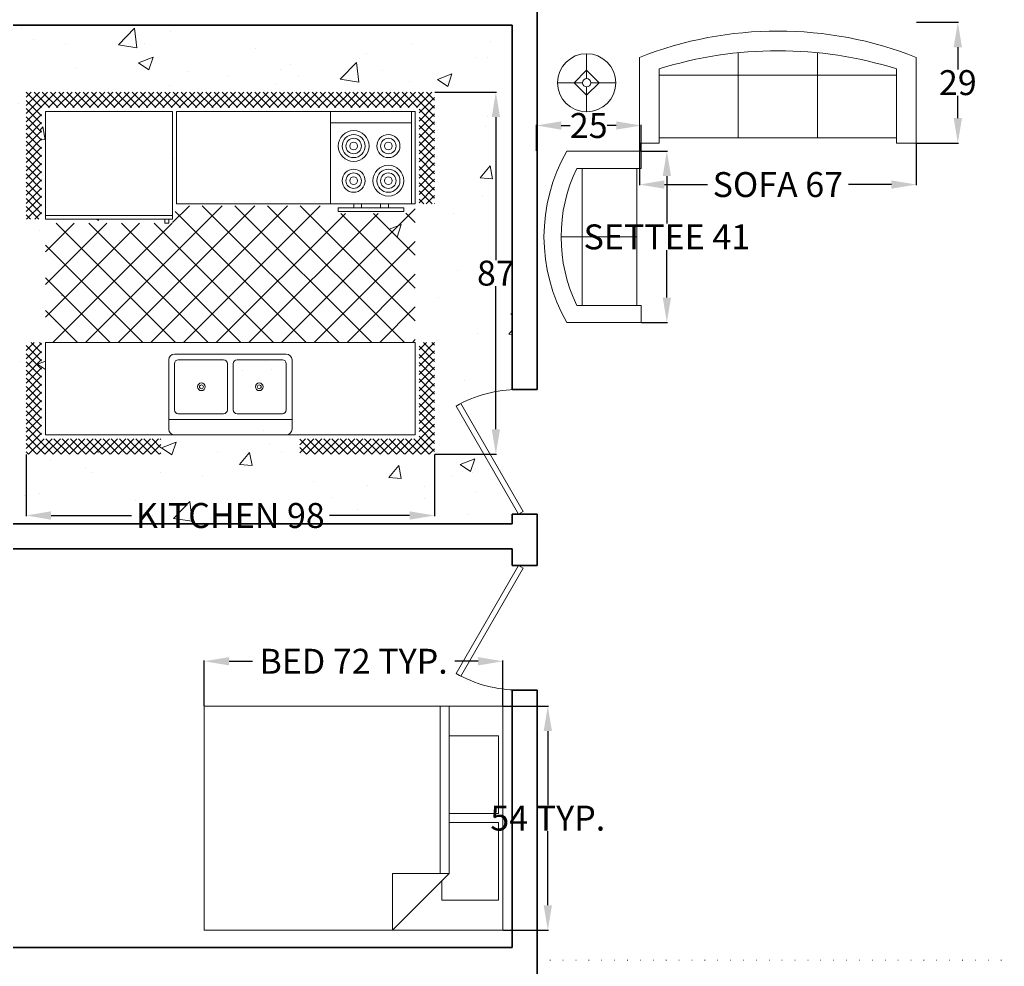
# Model space of a CAD drawing. Units: inches. Extents: x 910 to 1553, y 598 to 1516.
# Tile 4 of 6: x 1031 to 1268, y 1079 to 1307. Entities that reach past the tile are written whole.
import ezdxf

# ---------------------------------------------------------------- set-up
doc = ezdxf.new("R2010")
doc.units = ezdxf.units.IN
doc.header["$MEASUREMENT"] = 0
doc.linetypes.add('ACAD_ISO07W100', pattern=[3, 0, -3])
for name, color, linetype, lineweight in [('A-ANNO-DIMS', 2, 'Continuous', 18), ('A-FLOR-OVHD', 8, 'ACAD_ISO07W100', 13), ('A-FLOR-PATT', 252, 'Continuous', 13), ('doors', 2, 'Continuous', 18), ('furniture', 11, 'Continuous', 18), ('Inner wall', 230, 'Continuous', 35), ('kitchen', 90, 'Continuous', 18)]:
    doc.layers.add(name, color=color, linetype=linetype, lineweight=lineweight)
doc.styles.get("Standard").update_dxf_attribs({"font": 'arial.ttf'})
doc.dimstyles.get("Standard").update_dxf_attribs({"dimtxt": 6, "dimasz": 6, "dimexe": 0.18, "dimexo": 0.0625, "dimgap": 0.09, "dimtad": 0, "dimtih": 1, "dimtoh": 1, "dimdec": 0, "dimzin": 0, "dimdsep": 46, "dimlunit": 3, "dimtxsty": 'Standard', "dimcen": 0.09, "dimadec": 0, "dimazin": 0, "dimtfac": 1, "dimtdec": 0, "dimtofl": 0, "dimtmove": 0, "dimatfit": 3, "dimfxl": 1, "dimtolj": 1, "dimtzin": 0, "dimarcsym": 0})

# ---------------------------------------------------------------- blocks, each defined once
blk = doc.blocks.new('*U2')
for p, q in [((0, 0), (0, -6)), ((40, 0), (40, -6))]:
    blk.add_line(p, q)
blk.add_lwpolyline([(0, 0), (34.64, 20), (35.52, 18.48), (0.87, -1.52)], close=True)
blk.add_arc((0, 0), 40, 0, 30)
blk = doc.blocks.new('*U5')
for p, q in [((0, 0), (0, -6)), ((-40, 0), (-40, -6))]:
    blk.add_line(p, q)
blk.add_lwpolyline([(0, 0), (-34.64, 20), (-35.52, 18.48), (-0.88, -1.52)], close=True)
blk.add_arc((0, 0), 40, 150, 180)
blk = doc.blocks.new('Bed - Queen')
for p, q in [((0, -80.00003), (0, 0)), ((0, 0), (59.99999, 0)), ((59.99999, 0), (59.99999, -80.00003)), ((7.99999, -1.2), (28.79998, -1.2)), ((7.99999, -14.4), (7.99999, -1.2)), ((28.79998, -1.2), (28.79998, -14.4)), ((31.19999, -1.2), (51.99999, -1.2)), ((31.19999, -14.4), (31.19999, -1.2)), ((51.99999, -1.2), (51.99999, -16.4)), ((0, -14.4), (44.8, -14.4)), ((59.99999, -29.6), (44.8, -14.4)), ((44.8, -14.4), (44.8, -29.6)), ((44.8, -16.8), (0, -16.8)), ((51.99999, -16.4), (46.79936, -16.4)), ((44.8, -29.6), (59.99999, -29.6)), ((59.99999, -80.00003), (0, -80.00003))]:
    blk.add_line(p, q)
blk = doc.blocks.new('Kitchen Layout - 7 x 8 ft')
for p, q in [((-5, 81.32), (2.68, 89)), ((-5, 83.44), (0.56, 89)), ((-5, 85.56), (-1.56, 89)), ((-5, 87.68), (-3.68, 89)), ((-1, 84.97), (-5, 88.97)), ((1.09, 85), (-2.91, 89)), ((3.21, 85), (-0.79, 89)), ((0.81, 85), (4.81, 89)), ((5.34, 85), (1.34, 89)), ((2.93, 85), (6.93, 89)), ((7.46, 85), (3.46, 89)), ((5.05, 85), (9.05, 89)), ((9.58, 85), (5.58, 89)), ((7.17, 85), (11.17, 89)), ((11.7, 85), (7.7, 89)), ((9.29, 85), (13.29, 89)), ((13.82, 85), (9.82, 89)), ((11.41, 85), (15.41, 89)), ((15.94, 85), (11.94, 89)), ((13.53, 85), (17.53, 89)), ((18.06, 85), (14.06, 89)), ((15.65, 85), (19.65, 89)), ((20.18, 85), (16.18, 89)), ((17.78, 85), (21.78, 89)), ((22.31, 85), (18.31, 89)), ((19.9, 85), (23.9, 89)), ((24.43, 85), (20.43, 89)), ((22.02, 85), (26.02, 89)), ((26.55, 85), (22.55, 89)), ((24.14, 85), (28.14, 89)), ((28.67, 85), (24.67, 89)), ((26.26, 85), (30.26, 89)), ((30.79, 85), (26.79, 89)), ((28.38, 85), (32.38, 89)), ((32.91, 85), (28.91, 89)), ((30.5, 85), (34.5, 89)), ((35.03, 85), (31.03, 89)), ((32.63, 85), (36.63, 89)), ((37.16, 85), (33.16, 89)), ((34.75, 85), (38.75, 89)), ((39.28, 85), (35.28, 89)), ((36.87, 85), (40.87, 89)), ((41.4, 85), (37.4, 89)), ((38.99, 85), (42.99, 89)), ((43.52, 85), (39.52, 89)), ((41.11, 85), (45.11, 89)), ((45.64, 85), (41.64, 89)), ((43.23, 85), (47.23, 89)), ((47.76, 85), (43.76, 89)), ((45.35, 85), (49.35, 89)), ((49.88, 85), (45.88, 89)), ((47.47, 85), (51.47, 89)), ((52, 85), (48, 89)), ((49.6, 85), (53.6, 89)), ((54.13, 85), (50.13, 89)), ((51.72, 85), (55.72, 89)), ((56.25, 85), (52.25, 89)), ((53.84, 85), (57.84, 89)), ((58.37, 85), (54.37, 89)), ((55.96, 85), (59.96, 89)), ((60.49, 85), (56.49, 89)), ((58.08, 85), (62.08, 89)), ((62.61, 85), (58.61, 89)), ((60.2, 85), (64.2, 89)), ((64.73, 85), (60.73, 89)), ((62.32, 85), (66.32, 89)), ((66.85, 85), (62.85, 89)), ((64.45, 85), (68.45, 89)), ((68.97, 85), (64.97, 89)), ((66.57, 85), (70.57, 89)), ((71.1, 85), (67.1, 89)), ((68.69, 85), (72.69, 89)), ((73.22, 85), (69.22, 89)), ((70.81, 85), (74.81, 89)), ((75.34, 85), (71.34, 89)), ((72.93, 85), (76.93, 89)), ((77.46, 85), (73.46, 89)), ((75.05, 85), (79.05, 89)), ((79.58, 85), (75.58, 89)), ((77.17, 85), (81.17, 89)), ((81.7, 85), (77.7, 89)), ((79.29, 85), (83.29, 89)), ((83.82, 85), (79.82, 89)), ((81.42, 85), (85.42, 89)), ((85.95, 85), (81.95, 89)), ((83.54, 85), (87.54, 89)), ((88.07, 85), (84.07, 89)), ((85.66, 85), (89.66, 89)), ((90.19, 85), (86.19, 89)), ((87.78, 85), (91.78, 89)), ((92.31, 85), (88.31, 89)), ((89.9, 85), (93.9, 89)), ((94.43, 85), (90.43, 89)), ((92.02, 85), (96.02, 89)), ((96.55, 85), (92.55, 89)), ((94.14, 85), (98.14, 89)), ((101, 82.67), (94.67, 89)), ((96.27, 85), (100.27, 89)), ((101, 84.79), (96.79, 89)), ((97, 83.61), (101, 87.61)), ((101, 86.92), (98.92, 89)), ((-1, 82.85), (-5, 86.85)), ((-1, 80.73), (-5, 84.73)), ((97, 81.49), (101, 85.49)), ((101, 80.55), (97, 84.55)), ((-5, 79.19), (-1, 83.19)), ((-1, 78.61), (-5, 82.61)), ((34, 84), (96, 84)), ((34, 60), (34, 84)), ((96, 84), (96, 60)), ((97, 79.37), (101, 83.37)), ((101, 78.43), (97, 82.43)), ((-5, 77.07), (-1, 81.07)), ((-1, 76.49), (-5, 80.49)), ((74, 81), (95, 81)), ((97, 77.25), (101, 81.25)), ((101, 76.31), (97, 80.31)), ((-5, 74.95), (-1, 78.95)), ((-1, 74.36), (-5, 78.36)), ((-5, 72.83), (-1, 76.83)), ((97, 75.13), (101, 79.13)), ((101, 74.19), (97, 78.19)), ((97, 73.01), (101, 77.01)), ((-1, 72.24), (-5, 76.24)), ((-5, 70.71), (-1, 74.71)), ((-1, 70.12), (-5, 74.12)), ((101, 72.07), (97, 76.07)), ((97, 70.89), (101, 74.89)), ((-5, 68.59), (-1, 72.59)), ((-1, 68), (-5, 72)), ((101, 69.95), (97, 73.95)), ((97, 68.76), (101, 72.76)), ((101, 67.82), (97, 71.82)), ((-5, 66.47), (-1, 70.47)), ((-1, 65.88), (-5, 69.88)), ((97, 66.64), (101, 70.64)), ((101, 65.7), (97, 69.7)), ((-5, 64.35), (-1, 68.35)), ((-1, 63.76), (-5, 67.76)), ((97, 64.52), (101, 68.52)), ((101, 63.58), (97, 67.58)), ((-5, 62.22), (-1, 66.22)), ((-1, 61.64), (-5, 65.64)), ((-5, 60.1), (-1, 64.1)), ((97, 62.4), (101, 66.4)), ((101, 61.46), (97, 65.46)), ((97, 60.28), (101, 64.28)), ((-1, 59.52), (-5, 63.52)), ((-5, 57.98), (-1, 61.98)), ((-1, 57.39), (-5, 61.39)), ((100.34, 60), (97, 63.34)), ((98.84, 60), (101, 62.16)), ((-1.73, 56), (-5, 59.27)), ((-4.86, 56), (-1, 59.86)), ((10.4, 24), (45.9, 59.5)), ((18.88, 24), (54.38, 59.5)), ((27.37, 24), (62.87, 59.5)), ((33.03, 55.11), (37.41, 59.5)), ((96, 60), (34, 60)), ((35.85, 24), (71.35, 59.5)), ((76.2, 24), (40.7, 59.5)), ((84.68, 24), (49.18, 59.5)), ((93.17, 24), (57.67, 59.5)), ((96, 29.65), (66.15, 59.5)), ((80, 60), (80, 59)), ((82, 59), (82, 60)), ((87, 59), (87, 60)), ((89, 60), (89, 59)), ((98.22, 60), (97, 61.22)), ((100.96, 60), (101, 60.04)), ((-3.85, 56), (-5, 57.15)), ((-2.74, 56), (-1, 57.74)), ((0, 57), (33, 57)), ((67.71, 24), (33.68, 58.04)), ((44.34, 24), (77.84, 57.5)), ((52.82, 24), (86.32, 57.5)), ((61.31, 24), (96, 58.69)), ((96, 38.14), (76.64, 57.5)), ((96, 46.63), (85.13, 57.5)), ((96, 55.11), (93.57, 57.54)), ((0, 30.57), (24.43, 55)), ((0, 39.06), (15.94, 55)), ((0, 47.54), (7.46, 55)), ((1.91, 24), (32.91, 55)), ((33.77, 24), (2.77, 55)), ((42.26, 24), (11.26, 55)), ((50.74, 24), (19.74, 55)), ((59.23, 24), (28.23, 55)), ((31, 55), (31, 56)), ((32, 55), (31, 55)), ((32, 56), (32, 55)), ((25.29, 24), (0, 49.29)), ((69.79, 24), (96, 50.21)), ((78.28, 24), (96, 41.72)), ((16.8, 24), (0, 40.8)), ((86.76, 24), (96, 33.24)), ((8.32, 24), (0, 32.32)), ((-5, 21.92), (-2.92, 24)), ((-5, 19.8), (-1, 23.8)), ((-1, 19.21), (-5, 23.21)), ((-1, 21.33), (-3.67, 24)), ((-1, 23.45), (-1.55, 24)), ((0, 24), (96, 24)), ((0, 0), (0, 24)), ((95.25, 24), (96, 24.75)), ((96, 24), (96, 0)), ((97, 22.1), (98.9, 24)), ((97, 19.97), (101, 23.97)), ((101, 19.03), (97, 23.03)), ((101, 21.16), (98.16, 24)), ((101, 23.28), (100.28, 24)), ((-5, 17.68), (-1, 21.68)), ((-1, 17.09), (-5, 21.09)), ((97, 17.85), (101, 21.85)), ((101, 16.91), (97, 20.91)), ((-5, 15.55), (-1, 19.55)), ((-1, 14.97), (-5, 18.97)), ((47.25, 6.5), (47.25, 18.5)), ((48.75, 18.5), (48.75, 6.5)), ((97, 15.73), (101, 19.73)), ((101, 14.79), (97, 18.79)), ((-5, 13.43), (-1, 17.43)), ((-1, 12.85), (-5, 16.85)), ((97, 13.61), (101, 17.61)), ((101, 12.67), (97, 16.67)), ((97, 11.49), (101, 15.49)), ((-5, 11.31), (-1, 15.31)), ((-1, 10.73), (-5, 14.73)), ((-5, 9.19), (-1, 13.19)), ((101, 10.55), (97, 14.55)), ((97, 9.37), (101, 13.37)), ((-1, 8.6), (-5, 12.6)), ((-5, 7.07), (-1, 11.07)), ((-1, 6.48), (-5, 10.48)), ((101, 8.43), (97, 12.43)), ((97, 7.25), (101, 11.25)), ((101, 6.31), (97, 10.31)), ((-5, 4.95), (-1, 8.95)), ((-1, 4.36), (-5, 8.36)), ((97, 5.12), (101, 9.12)), ((101, 4.18), (97, 8.18)), ((-5, 2.83), (-1, 6.83)), ((-1, 2.24), (-5, 6.24)), ((97, 3), (101, 7)), ((101, 2.06), (97, 6.06)), ((-5, 0.71), (-1, 4.71)), ((-1, 0.12), (-5, 4.12)), ((-5, -1.42), (-1, 2.58)), ((64, 4), (32, 4)), ((93.24, -5), (101, 2.76)), ((97, 0.88), (101, 4.88)), ((101, -0.06), (97, 3.94)), ((2, -5), (-5, 2)), ((-5, -3.54), (-1, 0.46)), ((96, 0), (0, 0)), ((95.36, -5), (101, 0.64)), ((101, -2.18), (97, 1.82)), ((-0.12, -5), (-5, -0.12)), ((-2.25, -5), (-5, -2.25)), ((-4.34, -5), (-0.34, -1)), ((-2.22, -5), (1.78, -1)), ((-0.1, -5), (3.9, -1)), ((4.12, -5), (0.12, -1)), ((2.02, -5), (6.02, -1)), ((6.24, -5), (2.24, -1)), ((4.14, -5), (8.14, -1)), ((8.36, -5), (4.36, -1)), ((6.27, -5), (10.27, -1)), ((10.48, -5), (6.48, -1)), ((8.39, -5), (12.39, -1)), ((12.6, -5), (8.6, -1)), ((10.51, -5), (14.51, -1)), ((14.73, -5), (10.73, -1)), ((12.63, -5), (16.63, -1)), ((16.85, -5), (12.85, -1)), ((14.75, -5), (18.75, -1)), ((18.97, -5), (14.97, -1)), ((16.87, -5), (20.87, -1)), ((21.09, -5), (17.09, -1)), ((18.99, -5), (22.99, -1)), ((23.21, -5), (19.21, -1)), ((21.11, -5), (25.11, -1)), ((25.33, -5), (21.33, -1)), ((23.24, -5), (27.24, -1)), ((27.45, -5), (23.45, -1)), ((25.36, -5), (29.36, -1)), ((29.57, -5), (25.57, -1)), ((27.48, -5), (30, -2.48)), ((30, -3.3), (27.7, -1)), ((30, -1.18), (29.82, -1)), ((66, -2.54), (67.54, -1)), ((66, -4.66), (69.66, -1)), ((69.88, -5), (66, -1.12)), ((67.78, -5), (71.78, -1)), ((72, -5), (68, -1)), ((69.9, -5), (73.9, -1)), ((74.12, -5), (70.12, -1)), ((72.03, -5), (76.03, -1)), ((76.24, -5), (72.24, -1)), ((74.15, -5), (78.15, -1)), ((78.36, -5), (74.36, -1)), ((76.27, -5), (80.27, -1)), ((80.49, -5), (76.49, -1)), ((78.39, -5), (82.39, -1)), ((82.61, -5), (78.61, -1)), ((80.51, -5), (84.51, -1)), ((84.73, -5), (80.73, -1)), ((82.63, -5), (86.63, -1)), ((86.85, -5), (82.85, -1)), ((84.75, -5), (88.75, -1)), ((88.97, -5), (84.97, -1)), ((86.88, -5), (90.88, -1)), ((91.09, -5), (87.09, -1)), ((89, -5), (93, -1)), ((93.21, -5), (89.21, -1)), ((91.12, -5), (95.12, -1)), ((95.34, -5), (91.34, -1)), ((97.46, -5), (93.46, -1)), ((99.58, -5), (95.58, -1)), ((101, -4.3), (97, -0.3)), ((97.48, -5), (101, -1.48)), ((-4.37, -5), (-5, -4.37)), ((29.6, -5), (30, -4.6)), ((67.76, -5), (66, -3.24)), ((99.6, -5), (101, -3.6))]:
    blk.add_line(p, q)
for points in [[(0, 56), (0, 84), (33, 84), (33, 56)], [(74, 60), (74, 84), (95, 84), (95, 60)], [(76, 58), (76, 59), (93, 59), (93, 58)]]:
    blk.add_lwpolyline(points, close=True)
for points in [[(33.5, 21), (62.5, 21)], [(32, 1.5), (32, 19.5)], [(33.5, 6.5), (33.5, 18.5)], [(34.5, 19.5), (46.25, 19.5)], [(49.75, 19.5), (61.5, 19.5)], [(62.5, 18.5), (62.5, 6.5)], [(64, 19.5), (64, 1.5)], [(46.25, 5.5), (34.5, 5.5)], [(61.5, 5.5), (49.75, 5.5)], [(62.5, 0), (33.5, 0)]]:
    blk.add_lwpolyline(points)
for centre, radius in [((80, 75), 4), ((80, 75), 3), ((80, 75), 2), ((89, 75), 3), ((89, 75), 2), ((80, 75), 1), ((89, 75), 1), ((80, 66), 3), ((89, 66), 4), ((89, 66), 3), ((80, 66), 2), ((80, 66), 1), ((89, 66), 2), ((89, 66), 1), ((40.5, 12.5), 1), ((40.5, 12.5), 0.5), ((55.5, 12.5), 1), ((55.5, 12.5), 0.5)]:
    blk.add_circle(centre, radius)
for centre, radius, start, end in [((33.5, 19.5), 1.5, 90, 180), ((62.5, 19.5), 1.5, 0, 90), ((34.5, 18.5), 1, 90, 180), ((46.25, 18.5), 1, 0, 90), ((49.75, 18.5), 1, 90, 180), ((61.5, 18.5), 1, 0, 90), ((34.5, 6.5), 1, 180, 270), ((46.25, 6.5), 1, 270, 0), ((49.75, 6.5), 1, 180, 270), ((61.5, 6.5), 1, 270, 0), ((33.5, 1.5), 1.5, 180, 270), ((62.5, 1.5), 1.5, 270, 0)]:
    blk.add_arc(centre, radius, start, end)
blk = doc.blocks.new('Sofa - Roundback 7 ft.')
for p, q in [((-12.00002, -32.4421), (-12.00003, -6.5971)), ((11.99997, -32.4421), (11.99998, -6.5971)), ((-36.000027, -34), (-36.000027, -11.4696)), ((35.99998, -34), (35.99998, -11.4696)), ((-35.999844, -13.3819), (35.9998, -13.3819)), ((-36.000027, -32.4421), (35.99998, -32.4421))]:
    blk.add_line(p, q)
for points in [[(-36.000027, -34), (-42.000027, -34), (-42.000027, -8)], [(41.99998, -8), (41.99998, -34), (35.99998, -34)]]:
    blk.add_lwpolyline(points)
for centre, radius, start, end in [((0, -114.25), 114.25, 68.43141, 111.5686), ((-0.00001, -127.1968), 121.1968, 72.72033, 107.2797)]:
    blk.add_arc(centre, radius, start, end)
blk = doc.blocks.new('Sofa - Roundback Loveseat 5 ft.')
for p, q in [((0, -32.44198), (0, -5.99998)), ((-24, -33.99998), (-24, -11.46958)), ((-23.9998, -13.38178), (23.99986, -13.38178)), ((24.00004, -33.99998), (24.00004, -11.46958)), ((-24, -32.44198), (24.00004, -32.44198))]:
    blk.add_line(p, q)
for points in [[(-24, -33.99998), (-30, -33.99998), (-30, -7.99998)], [(30.00004, -7.99998), (30.00004, -33.99998), (24.00004, -33.99998)]]:
    blk.add_lwpolyline(points)
for centre, radius, start, end in [((0, -60.24998), 60.24998, 60.13715, 119.8628), ((0, -61.38438), 55.38444, 64.32083, 115.6792)]:
    blk.add_arc(centre, radius, start, end)
blk = doc.blocks.new('Lamp - Table')
for p, q in [((0, 7), (0, 1)), ((0, 3), (-3, 0)), ((3, 0), (0, 3)), ((-1, 0), (-7, 0)), ((-3, 0), (0, -3)), ((0, -3), (3, 0)), ((1, 0), (7, 0)), ((0, -1), (0, -7))]:
    blk.add_line(p, q)
for radius in [7, 1]:
    blk.add_circle((0, 0), radius)
blk = doc.blocks.new('*D27')
at = {"layer": 'A-ANNO-DIMS', "color": 0, "lineweight": -2, "transparency": 16777216}
for p, q in [((1075.61, 1142.16), (1075.61, 1153.06)), ((1081.61, 1152.88), (1087.21, 1152.88)), ((1141.5, 1152.88), (1135.9, 1152.88)), ((1147.5, 1142.16), (1147.5, 1153.06))]:
    blk.add_line(p, q, dxfattribs=at)
for points in [[(1081.61, 1153.88), (1081.61, 1151.88), (1075.61, 1152.88)], [(1141.5, 1153.88), (1141.5, 1151.88), (1147.5, 1152.88)]]:
    blk.add_solid(points, dxfattribs=at)
at = {"layer": 'Defpoints', "color": 0, "lineweight": -2, "transparency": 16777216}
for p in [(1147.5, 1152.88), (1075.61, 1142.09), (1147.5, 1142.09)]:
    blk.add_point(p, dxfattribs=at)
at = {"layer": 'A-ANNO-DIMS', "color": 0, "transparency": 16777216, "insert": (1111.56, 1152.88), "char_height": 6, "attachment_point": 5}
blk.add_mtext('\\A1;BED 72 TYP.', dxfattribs=at)
blk = doc.blocks.new('*D28')
at = {"layer": 'A-ANNO-DIMS', "color": 0, "lineweight": -2, "transparency": 16777216}
for p, q in [((1147.56, 1142.09), (1158.46, 1142.09)), ((1158.28, 1136.09), (1158.28, 1118.28)), ((1158.28, 1094.18), (1158.28, 1112)), ((1147.56, 1088.18), (1158.46, 1088.18))]:
    blk.add_line(p, q, dxfattribs=at)
for points in [[(1157.28, 1136.09), (1159.28, 1136.09), (1158.28, 1142.09)], [(1157.28, 1094.18), (1159.28, 1094.18), (1158.28, 1088.18)]]:
    blk.add_solid(points, dxfattribs=at)
at = {"layer": 'Defpoints', "color": 0, "lineweight": -2, "transparency": 16777216}
for p in [(1147.5, 1142.09), (1147.5, 1088.18), (1158.28, 1088.18)]:
    blk.add_point(p, dxfattribs=at)
at = {"layer": 'A-ANNO-DIMS', "color": 0, "transparency": 16777216, "insert": (1158.28, 1115.14), "char_height": 6, "attachment_point": 5}
blk.add_mtext('\\A1;54 TYP.', dxfattribs=at)
blk = doc.blocks.new('*D43')
at = {"layer": 'A-ANNO-DIMS', "color": 0, "lineweight": -2, "transparency": 16777216}
for p, q in [((1180.8, 1275.63), (1187.1, 1275.63)), ((1186.92, 1269.63), (1186.92, 1258.2)), ((1186.92, 1240.39), (1186.92, 1251.81)), ((1180.8, 1234.39), (1187.1, 1234.39))]:
    blk.add_line(p, q, dxfattribs=at)
for points in [[(1185.92, 1269.63), (1187.92, 1269.63), (1186.92, 1275.63)], [(1185.92, 1240.39), (1187.92, 1240.39), (1186.92, 1234.39)]]:
    blk.add_solid(points, dxfattribs=at)
at = {"layer": 'Defpoints', "color": 0, "lineweight": -2, "transparency": 16777216}
for p in [(1180.73, 1275.63), (1186.92, 1275.63), (1180.73, 1234.39)]:
    blk.add_point(p, dxfattribs=at)
at = {"layer": 'A-ANNO-DIMS', "color": 0, "transparency": 16777216, "insert": (1186.92, 1255.01), "char_height": 6, "attachment_point": 5}
blk.add_mtext('\\A1;SETTEE 41', dxfattribs=at)
blk = doc.blocks.new('*D44')
at = {"layer": 'A-ANNO-DIMS', "color": 0, "lineweight": -2, "transparency": 16777216}
for p, q in [((1155.53, 1275.69), (1155.53, 1281.99)), ((1161.53, 1281.81), (1163.67, 1281.81)), ((1174.73, 1281.81), (1172.59, 1281.81)), ((1180.73, 1275.69), (1180.73, 1281.99))]:
    blk.add_line(p, q, dxfattribs=at)
for points in [[(1161.53, 1282.81), (1161.53, 1280.81), (1155.53, 1281.81)], [(1174.73, 1282.81), (1174.73, 1280.81), (1180.73, 1281.81)]]:
    blk.add_solid(points, dxfattribs=at)
at = {"layer": 'Defpoints', "color": 0, "lineweight": -2, "transparency": 16777216}
for p in [(1155.53, 1281.81), (1155.53, 1275.63), (1180.73, 1275.63)]:
    blk.add_point(p, dxfattribs=at)
at = {"layer": 'A-ANNO-DIMS', "color": 0, "transparency": 16777216, "insert": (1168.13, 1281.81), "char_height": 6, "attachment_point": 5}
blk.add_mtext('\\A1;25', dxfattribs=at)
blk = doc.blocks.new('*D49')
at = {"layer": 'A-ANNO-DIMS', "color": 0, "lineweight": -2, "transparency": 16777216}
for p, q in [((1032.78, 1202.64), (1032.78, 1187.78)), ((1131.05, 1202.64), (1131.05, 1187.78)), ((1038.78, 1187.96), (1058.1, 1187.96)), ((1125.05, 1187.96), (1105.73, 1187.96))]:
    blk.add_line(p, q, dxfattribs=at)
for points in [[(1038.78, 1188.96), (1038.78, 1186.96), (1032.78, 1187.96)], [(1125.05, 1188.96), (1125.05, 1186.96), (1131.05, 1187.96)]]:
    blk.add_solid(points, dxfattribs=at)
at = {"layer": 'Defpoints', "color": 0, "lineweight": -2, "transparency": 16777216}
for p in [(1032.78, 1202.71), (1131.05, 1202.71), (1131.05, 1187.96)]:
    blk.add_point(p, dxfattribs=at)
at = {"layer": 'A-ANNO-DIMS', "color": 0, "transparency": 16777216, "insert": (1081.91, 1187.96), "char_height": 6, "attachment_point": 5}
blk.add_mtext('\\A1;KITCHEN 98', dxfattribs=at)
blk = doc.blocks.new('*D50')
at = {"layer": 'A-ANNO-DIMS', "color": 0, "lineweight": -2, "transparency": 16777216}
for p, q in [((1131.11, 1289.85), (1145.97, 1289.85)), ((1145.79, 1283.85), (1145.79, 1249.43)), ((1145.79, 1208.71), (1145.79, 1243.12)), ((1131.11, 1202.71), (1145.97, 1202.71))]:
    blk.add_line(p, q, dxfattribs=at)
for points in [[(1144.79, 1283.85), (1146.79, 1283.85), (1145.79, 1289.85)], [(1144.79, 1208.71), (1146.79, 1208.71), (1145.79, 1202.71)]]:
    blk.add_solid(points, dxfattribs=at)
at = {"layer": 'Defpoints', "color": 0, "lineweight": -2, "transparency": 16777216}
for p in [(1131.05, 1289.85), (1145.79, 1289.85), (1131.05, 1202.71)]:
    blk.add_point(p, dxfattribs=at)
at = {"layer": 'A-ANNO-DIMS', "color": 0, "transparency": 16777216, "insert": (1145.79, 1246.28), "char_height": 6, "attachment_point": 5}
blk.add_mtext('\\A1;87', dxfattribs=at)
blk = doc.blocks.new('*D51')
at = {"layer": 'A-ANNO-DIMS', "color": 0, "lineweight": -2, "transparency": 16777216}
for p, q in [((1180.32, 1277.53), (1180.32, 1267.42)), ((1246.93, 1277.53), (1246.93, 1267.42)), ((1186.32, 1267.6), (1196.68, 1267.6)), ((1240.93, 1267.6), (1230.58, 1267.6))]:
    blk.add_line(p, q, dxfattribs=at)
for points in [[(1186.32, 1268.6), (1186.32, 1266.6), (1180.32, 1267.6)], [(1240.93, 1268.6), (1240.93, 1266.6), (1246.93, 1267.6)]]:
    blk.add_solid(points, dxfattribs=at)
at = {"layer": 'Defpoints', "color": 0, "lineweight": -2, "transparency": 16777216}
for p in [(1180.32, 1277.59), (1246.93, 1277.59), (1246.93, 1267.6)]:
    blk.add_point(p, dxfattribs=at)
at = {"layer": 'A-ANNO-DIMS', "color": 0, "transparency": 16777216, "insert": (1213.63, 1267.6), "char_height": 6, "attachment_point": 5}
blk.add_mtext('\\A1;SOFA 67', dxfattribs=at)
blk = doc.blocks.new('*D52')
at = {"layer": 'A-ANNO-DIMS', "color": 0, "lineweight": -2, "transparency": 16777216}
for p, q in [((1247, 1306.66), (1257.1, 1306.66)), ((1256.92, 1300.66), (1256.92, 1295.28)), ((1256.92, 1283.59), (1256.92, 1288.97)), ((1247, 1277.59), (1257.1, 1277.59))]:
    blk.add_line(p, q, dxfattribs=at)
for points in [[(1255.92, 1300.66), (1257.92, 1300.66), (1256.92, 1306.66)], [(1255.92, 1283.59), (1257.92, 1283.59), (1256.92, 1277.59)]]:
    blk.add_solid(points, dxfattribs=at)
at = {"layer": 'Defpoints', "color": 0, "lineweight": -2, "transparency": 16777216}
for p in [(1246.93, 1306.66), (1256.92, 1306.66), (1246.93, 1277.59)]:
    blk.add_point(p, dxfattribs=at)
at = {"layer": 'A-ANNO-DIMS', "color": 0, "transparency": 16777216, "insert": (1256.92, 1292.13), "char_height": 6, "attachment_point": 5}
blk.add_mtext('\\A1;29', dxfattribs=at)

msp = doc.modelspace()

# ---------------------------------------------------------------- hatches: boundary and pattern name
at = {"layer": 'A-FLOR-PATT'}
h = msp.add_hatch(dxfattribs=at)
h.set_pattern_fill('AR-CONC', color=256, scale=5)
h.paths.add_polyline_path([(1149.7, 1305.969), (1029.7, 1305.969), (1023.7, 1305.969), (963.7, 1305.969), (963.7, 1233.969), (1023.7, 1233.969), (1029.7, 1233.969), (1029.7, 1185.969), (1149.7, 1185.969), (1149.7, 1188.289), (1151.2, 1188.289), (1136.2, 1214.269), (1137.337, 1214.926), (1137.352, 1214.901, -0.107869), (1149.7, 1218.251)])
h.paths.add_polyline_path([(1037.415, 1285.215), (1068.009, 1285.215), (1068.009, 1259.257), (1067.082, 1259.257), (1067.082, 1258.33), (1066.155, 1258.33), (1066.155, 1259.257), (1037.415, 1259.257)], flags=16)
h.paths.add_polyline_path([(1033.378, 1259.726), (1032.395, 1260.709), (1033.378, 1261.693), (1032.395, 1262.676), (1033.378, 1263.659), (1032.395, 1264.642), (1033.378, 1265.626), (1032.395, 1266.609), (1033.378, 1267.592), (1032.395, 1268.576), (1033.378, 1269.559), (1032.395, 1270.542), (1033.378, 1271.526), (1032.395, 1272.509), (1033.378, 1273.492), (1032.395, 1274.476), (1033.378, 1275.459), (1032.395, 1276.442), (1033.378, 1277.426), (1032.395, 1278.409), (1033.378, 1279.392), (1032.395, 1280.376), (1033.378, 1281.359), (1032.395, 1282.342), (1033.378, 1283.326), (1032.395, 1284.309), (1033.378, 1285.292), (1032.395, 1286.275), (1033.378, 1287.259), (1032.395, 1288.242), (1034.362, 1290.209), (1035.345, 1289.225), (1036.328, 1290.209), (1037.312, 1289.225), (1038.295, 1290.209), (1039.278, 1289.225), (1040.262, 1290.209), (1041.245, 1289.225), (1042.228, 1290.209), (1043.212, 1289.225), (1044.195, 1290.209), (1045.178, 1289.225), (1046.162, 1290.209), (1047.145, 1289.225), (1048.128, 1290.209), (1049.111, 1289.225), (1050.095, 1290.209), (1051.078, 1289.225), (1052.061, 1290.209), (1053.045, 1289.225), (1054.028, 1290.209), (1055.011, 1289.225), (1055.995, 1290.209), (1056.978, 1289.225), (1057.961, 1290.209), (1058.945, 1289.225), (1059.928, 1290.209), (1060.911, 1289.225), (1061.895, 1290.209), (1062.878, 1289.225), (1063.861, 1290.209), (1064.845, 1289.225), (1065.828, 1290.209), (1066.811, 1289.225), (1067.795, 1290.209), (1068.778, 1289.225), (1069.761, 1290.209), (1070.745, 1289.225), (1071.728, 1290.209), (1072.711, 1289.225), (1073.694, 1290.209), (1074.678, 1289.225), (1075.661, 1290.209), (1076.644, 1289.225), (1077.628, 1290.209), (1078.611, 1289.225), (1079.594, 1290.209), (1080.578, 1289.225), (1081.561, 1290.209), (1082.544, 1289.225), (1083.528, 1290.209), (1084.511, 1289.225), (1085.494, 1290.209), (1086.478, 1289.225), (1087.461, 1290.209), (1088.444, 1289.225), (1089.428, 1290.209), (1090.411, 1289.225), (1091.394, 1290.209), (1092.378, 1289.225), (1093.361, 1290.209), (1094.344, 1289.225), (1095.327, 1290.209), (1096.311, 1289.225), (1097.294, 1290.209), (1098.277, 1289.225), (1099.261, 1290.209), (1100.244, 1289.225), (1101.227, 1290.209), (1102.211, 1289.225), (1103.194, 1290.209), (1104.177, 1289.225), (1105.161, 1290.209), (1106.144, 1289.225), (1107.127, 1290.209), (1108.111, 1289.225), (1109.094, 1290.209), (1110.077, 1289.225), (1111.061, 1290.209), (1112.044, 1289.225), (1113.027, 1290.209), (1114.011, 1289.225), (1114.994, 1290.209), (1115.977, 1289.225), (1116.961, 1290.209), (1117.944, 1289.225), (1118.927, 1290.209), (1119.91, 1289.225), (1120.894, 1290.209), (1121.877, 1289.225), (1122.86, 1290.209), (1123.844, 1289.225), (1124.827, 1290.209), (1125.81, 1289.225), (1126.794, 1290.209), (1127.777, 1289.225), (1128.76, 1290.209), (1130.727, 1288.242), (1129.744, 1287.259), (1130.727, 1286.275), (1129.744, 1285.292), (1130.727, 1284.309), (1129.744, 1283.326), (1130.727, 1282.342), (1129.744, 1281.359), (1130.727, 1280.376), (1129.744, 1279.392), (1130.727, 1278.409), (1129.744, 1277.426), (1130.727, 1276.442), (1129.744, 1275.459), (1130.727, 1274.476), (1129.744, 1273.492), (1130.727, 1272.509), (1129.744, 1271.526), (1130.727, 1270.542), (1129.744, 1269.559), (1130.727, 1268.576), (1129.744, 1267.592), (1130.727, 1266.609), (1129.744, 1265.626), (1130.727, 1264.642), (1128.76, 1262.676), (1127.777, 1263.659), (1128.76, 1264.642), (1127.777, 1265.626), (1128.76, 1266.609), (1127.777, 1267.592), (1128.76, 1268.576), (1127.777, 1269.559), (1128.76, 1270.542), (1127.777, 1271.526), (1128.76, 1272.509), (1127.777, 1273.492), (1128.76, 1274.476), (1127.777, 1275.459), (1128.76, 1276.442), (1127.777, 1277.426), (1128.76, 1278.409), (1127.777, 1279.392), (1128.76, 1280.376), (1127.777, 1281.359), (1128.76, 1282.342), (1127.777, 1283.326), (1128.76, 1284.309), (1127.342, 1285.727), (1125.81, 1287.259), (1124.827, 1286.275), (1123.844, 1287.259), (1122.86, 1286.275), (1121.877, 1287.259), (1120.894, 1286.275), (1119.91, 1287.259), (1118.927, 1286.275), (1117.944, 1287.259), (1116.961, 1286.275), (1115.977, 1287.259), (1114.994, 1286.275), (1114.011, 1287.259), (1113.027, 1286.275), (1112.044, 1287.259), (1111.061, 1286.275), (1110.077, 1287.259), (1109.094, 1286.275), (1108.111, 1287.259), (1107.127, 1286.275), (1106.144, 1287.259), (1105.161, 1286.275), (1104.177, 1287.259), (1103.194, 1286.275), (1102.211, 1287.259), (1101.227, 1286.275), (1100.244, 1287.259), (1099.261, 1286.275), (1098.277, 1287.259), (1097.294, 1286.275), (1096.311, 1287.259), (1095.327, 1286.275), (1094.344, 1287.259), (1093.361, 1286.275), (1092.378, 1287.259), (1091.394, 1286.275), (1090.411, 1287.259), (1089.428, 1286.275), (1088.444, 1287.259), (1087.461, 1286.275), (1086.478, 1287.259), (1085.494, 1286.275), (1084.511, 1287.259), (1083.528, 1286.275), (1082.544, 1287.259), (1081.561, 1286.275), (1080.578, 1287.259), (1079.594, 1286.275), (1078.611, 1287.259), (1077.628, 1286.275), (1076.644, 1287.259), (1075.661, 1286.275), (1074.678, 1287.259), (1073.694, 1286.275), (1072.711, 1287.259), (1071.728, 1286.275), (1070.745, 1287.259), (1069.761, 1286.275), (1068.778, 1287.259), (1067.795, 1286.275), (1066.811, 1287.259), (1065.828, 1286.275), (1064.845, 1287.259), (1063.861, 1286.275), (1062.878, 1287.259), (1061.895, 1286.275), (1060.911, 1287.259), (1059.928, 1286.275), (1058.945, 1287.259), (1057.961, 1286.275), (1056.978, 1287.259), (1055.995, 1286.275), (1055.011, 1287.259), (1054.028, 1286.275), (1053.045, 1287.259), (1052.061, 1286.275), (1051.078, 1287.259), (1050.095, 1286.275), (1049.111, 1287.259), (1048.128, 1286.275), (1047.145, 1287.259), (1046.162, 1286.275), (1045.178, 1287.259), (1044.195, 1286.275), (1043.212, 1287.259), (1042.228, 1286.275), (1041.245, 1287.259), (1040.262, 1286.275), (1039.278, 1287.259), (1038.295, 1286.275), (1037.312, 1287.259), (1035.345, 1285.292), (1036.328, 1284.309), (1035.345, 1283.326), (1036.328, 1282.342), (1035.345, 1281.359), (1036.328, 1280.376), (1035.345, 1279.392), (1036.328, 1278.409), (1035.345, 1277.426), (1036.328, 1276.442), (1035.345, 1275.459), (1036.328, 1274.476), (1035.345, 1273.492), (1036.328, 1272.509), (1035.345, 1271.526), (1036.328, 1270.542), (1035.345, 1269.559), (1036.328, 1268.576), (1035.345, 1267.592), (1036.328, 1266.609), (1035.345, 1265.626), (1036.328, 1264.642), (1035.345, 1263.659), (1036.328, 1262.676), (1035.345, 1261.693), (1036.328, 1260.709), (1035.345, 1259.726), (1034.362, 1260.709)], flags=16)
h.paths.add_polyline_path([(1107.873, 1261.111), (1107.873, 1262.038), (1111.582, 1262.038), (1111.582, 1262.965), (1106.019, 1262.965), (1068.936, 1262.965), (1068.936, 1285.215), (1126.415, 1285.215), (1126.415, 1262.965), (1125.488, 1262.965), (1125.488, 1262.965), (1119.925, 1262.965), (1119.925, 1262.038), (1123.634, 1262.038), (1123.634, 1261.111)], flags=16)
h.paths.add_polyline_path([(1038.223, 1252.226), (1042.156, 1256.159), (1046.09, 1252.226), (1050.023, 1256.159), (1053.956, 1252.226), (1057.889, 1256.159), (1061.823, 1252.226), (1067.927, 1258.33), (1069.689, 1260.092), (1073.622, 1256.159), (1077.556, 1260.092), (1081.489, 1256.159), (1085.422, 1260.092), (1089.356, 1256.159), (1093.289, 1260.092), (1097.222, 1256.159), (1101.155, 1260.092), (1105.089, 1256.159), (1109.022, 1260.092), (1112.955, 1256.159), (1116.889, 1260.092), (1124.755, 1252.226), (1120.822, 1248.292), (1124.755, 1244.359), (1120.822, 1240.426), (1124.755, 1236.493), (1120.822, 1232.559), (1123.791, 1229.59), (1126.415, 1229.59), (1126.415, 1207.34), (1037.415, 1207.34), (1037.415, 1229.59), (1039.187, 1229.59), (1042.156, 1232.559), (1038.223, 1236.493), (1042.156, 1240.426), (1038.223, 1244.359), (1042.156, 1248.292)], flags=16)
h.paths.add_polyline_path([(1036.328, 1227.276), (1035.345, 1226.293), (1036.328, 1225.31), (1035.345, 1224.326), (1036.328, 1223.343), (1035.345, 1222.36), (1036.328, 1221.376), (1035.345, 1220.393), (1036.328, 1219.41), (1035.345, 1218.426), (1036.328, 1217.443), (1035.345, 1216.46), (1036.328, 1215.476), (1035.345, 1214.493), (1036.328, 1213.51), (1035.345, 1212.527), (1036.328, 1211.543), (1035.345, 1210.56), (1036.328, 1209.577), (1035.345, 1208.593), (1036.328, 1207.61), (1035.345, 1206.627), (1036.328, 1205.643), (1037.312, 1206.627), (1038.295, 1205.643), (1039.278, 1206.627), (1040.262, 1205.643), (1041.245, 1206.627), (1042.228, 1205.643), (1043.212, 1206.627), (1044.195, 1205.643), (1045.178, 1206.627), (1046.162, 1205.643), (1047.145, 1206.627), (1048.128, 1205.643), (1049.111, 1206.627), (1050.095, 1205.643), (1051.078, 1206.627), (1052.061, 1205.643), (1053.045, 1206.627), (1054.028, 1205.643), (1055.011, 1206.627), (1055.995, 1205.643), (1056.978, 1206.627), (1057.961, 1205.643), (1058.945, 1206.627), (1059.928, 1205.643), (1060.911, 1206.627), (1061.895, 1205.643), (1062.878, 1206.627), (1064.845, 1204.66), (1062.878, 1202.693), (1061.895, 1203.677), (1060.911, 1202.693), (1059.928, 1203.677), (1058.945, 1202.693), (1057.961, 1203.677), (1056.978, 1202.693), (1055.995, 1203.677), (1055.011, 1202.693), (1054.028, 1203.677), (1053.045, 1202.693), (1052.061, 1203.677), (1051.078, 1202.693), (1050.095, 1203.677), (1049.111, 1202.693), (1048.128, 1203.677), (1047.145, 1202.693), (1046.162, 1203.677), (1045.178, 1202.693), (1044.195, 1203.677), (1043.212, 1202.693), (1042.228, 1203.677), (1041.245, 1202.693), (1040.262, 1203.677), (1039.278, 1202.693), (1038.295, 1203.677), (1037.312, 1202.693), (1036.328, 1203.677), (1035.345, 1202.693), (1034.362, 1203.677), (1033.378, 1202.693), (1032.395, 1203.677), (1033.378, 1204.66), (1032.395, 1205.643), (1033.378, 1206.627), (1032.395, 1207.61), (1033.378, 1208.593), (1032.395, 1209.577), (1033.378, 1210.56), (1032.395, 1211.543), (1033.378, 1212.527), (1032.395, 1213.51), (1033.378, 1214.493), (1032.395, 1215.476), (1033.378, 1216.46), (1032.395, 1217.443), (1033.378, 1218.426), (1032.395, 1219.41), (1033.378, 1220.393), (1032.395, 1221.376), (1033.378, 1222.36), (1032.395, 1223.343), (1033.378, 1224.326), (1032.395, 1225.31), (1033.378, 1226.293), (1032.395, 1227.276), (1034.362, 1229.243)], flags=16)
h.paths.add_polyline_path([(1068.472, 1226.809), (1095.358, 1226.809, -0.4142136), (1096.748, 1225.419), (1096.748, 1208.731, -0.4142136), (1095.358, 1207.34), (1068.472, 1207.34, -0.4142136), (1067.082, 1208.731), (1067.082, 1225.419, -0.4142136)], flags=16)
h.paths.add_polyline_path([(1068.472, 1224.491, -0.4142136), (1069.399, 1225.419), (1080.293, 1225.419, -0.4142136), (1081.22, 1224.491), (1081.22, 1213.366, -0.4142136), (1080.293, 1212.439), (1069.399, 1212.439, -0.4142136), (1068.472, 1213.366)], flags=0)
h.paths.add_polyline_path([(1074.498, 1218.929, -1), (1075.425, 1218.929, -1)], flags=0)
h.paths.add_polyline_path([(1082.61, 1224.491, -0.4142136), (1083.537, 1225.419), (1094.431, 1225.419, -0.4142136), (1095.358, 1224.491), (1095.358, 1213.366, -0.4142136), (1094.431, 1212.439), (1083.537, 1212.439, -0.4142136), (1082.61, 1213.366)], flags=0)
h.paths.add_polyline_path([(1088.405, 1218.929, -1), (1089.332, 1218.929, -1)], flags=0)
h.paths.add_polyline_path([(1114.363, 1268.528, -1), (1108.8, 1268.528, -1)], flags=0)
h.paths.add_polyline_path([(1107.873, 1276.872, -1), (1115.29, 1276.872, -1)], flags=0)
h.paths.add_polyline_path([(1113.436, 1268.528, -1), (1109.727, 1268.528, -1)], flags=0)
h.paths.add_polyline_path([(1114.363, 1276.872, -1), (1108.8, 1276.872, -1)], flags=0)
h.paths.add_polyline_path([(1112.509, 1268.528, -1), (1110.655, 1268.528, -1)], flags=0)
h.paths.add_polyline_path([(1113.436, 1276.872, -1), (1109.727, 1276.872, -1)], flags=0)
h.paths.add_polyline_path([(1112.509, 1276.872, -1), (1110.655, 1276.872, -1)], flags=0)
h.paths.add_polyline_path([(1100.244, 1206.627), (1101.227, 1205.643), (1102.211, 1206.627), (1103.194, 1205.643), (1104.177, 1206.627), (1105.161, 1205.643), (1106.144, 1206.627), (1107.127, 1205.643), (1108.111, 1206.627), (1109.094, 1205.643), (1110.077, 1206.627), (1111.061, 1205.643), (1112.044, 1206.627), (1113.027, 1205.643), (1114.011, 1206.627), (1114.994, 1205.643), (1115.977, 1206.627), (1116.961, 1205.643), (1117.944, 1206.627), (1118.927, 1205.643), (1119.91, 1206.627), (1120.894, 1205.643), (1121.877, 1206.627), (1122.86, 1205.643), (1123.844, 1206.627), (1124.827, 1205.643), (1125.81, 1206.627), (1126.794, 1205.643), (1128.76, 1207.61), (1127.777, 1208.593), (1128.76, 1209.577), (1127.777, 1210.56), (1128.76, 1211.543), (1127.777, 1212.527), (1128.76, 1213.51), (1127.777, 1214.493), (1128.76, 1215.476), (1127.777, 1216.46), (1128.76, 1217.443), (1127.777, 1218.426), (1128.76, 1219.41), (1127.777, 1220.393), (1128.76, 1221.376), (1127.777, 1222.36), (1128.76, 1223.343), (1127.777, 1224.326), (1128.76, 1225.31), (1127.777, 1226.293), (1128.76, 1227.276), (1127.777, 1228.26), (1128.76, 1229.243), (1130.727, 1227.276), (1129.744, 1226.293), (1130.727, 1225.31), (1129.744, 1224.326), (1130.727, 1223.343), (1129.744, 1222.36), (1130.727, 1221.376), (1129.744, 1220.393), (1130.727, 1219.41), (1129.744, 1218.426), (1130.727, 1217.443), (1129.744, 1216.46), (1130.727, 1215.476), (1129.744, 1214.493), (1130.727, 1213.51), (1129.744, 1212.527), (1130.727, 1211.543), (1129.744, 1210.56), (1130.727, 1209.577), (1129.744, 1208.593), (1130.727, 1207.61), (1129.744, 1206.627), (1130.727, 1205.643), (1129.744, 1204.66), (1130.727, 1203.677), (1129.744, 1202.693), (1128.76, 1203.677), (1127.777, 1202.693), (1126.794, 1203.677), (1125.81, 1202.693), (1124.827, 1203.677), (1123.844, 1202.693), (1122.86, 1203.677), (1121.877, 1202.693), (1120.894, 1203.677), (1119.91, 1202.693), (1118.927, 1203.677), (1117.944, 1202.693), (1116.961, 1203.677), (1115.977, 1202.693), (1114.994, 1203.677), (1114.011, 1202.693), (1113.027, 1203.677), (1112.044, 1202.693), (1111.061, 1203.677), (1110.077, 1202.693), (1109.094, 1203.677), (1108.111, 1202.693), (1107.127, 1203.677), (1106.144, 1202.693), (1105.161, 1203.677), (1104.177, 1202.693), (1103.194, 1203.677), (1102.211, 1202.693), (1101.227, 1203.677), (1100.244, 1202.693), (1098.277, 1204.66)], flags=16)
h.paths.add_polyline_path([(1123.634, 1268.528, -1), (1116.217, 1268.528, -1)], flags=0)
h.paths.add_polyline_path([(1122.707, 1268.528, -1), (1117.144, 1268.528, -1)], flags=0)
h.paths.add_polyline_path([(1121.779, 1268.528, -1), (1118.071, 1268.528, -1)], flags=0)
h.paths.add_polyline_path([(1122.707, 1276.872, -1), (1117.144, 1276.872, -1)], flags=0)
h.paths.add_polyline_path([(1120.852, 1268.528, -1), (1118.998, 1268.528, -1)], flags=0)
h.paths.add_polyline_path([(1121.779, 1276.872, -1), (1118.071, 1276.872, -1)], flags=0)
h.paths.add_polyline_path([(1120.852, 1276.872, -1), (1118.998, 1276.872, -1)], flags=0)

# ---------------------------------------------------------------- linework, layer by layer
at = {"layer": 'A-FLOR-OVHD'}
msp.add_line((1155.7, 1080.969), (1281.7, 1080.969), dxfattribs=at)
at = {"layer": 'Inner wall'}
for p, q in [((1155.7, 1313.296), (1155.7, 1218.289)), ((1155.7, 1313.296), (1155.7, 1218.289)), ((1149.7, 1305.969), (1029.7, 1305.969)), ((1149.7, 1305.969), (1149.7, 1218.289)), ((1149.7, 1188.289), (1149.7, 1185.969)), ((1155.7, 1188.289), (1155.7, 1185.969)), ((1155.7, 1188.289), (1155.7, 1175.953)), ((1155.7, 1188.289), (1155.7, 1175.953)), ((1149.7, 1185.969), (1029.7, 1185.969)), ((1149.7, 1179.969), (1029.7, 1179.969)), ((1149.7, 1179.969), (1149.7, 1175.953)), ((1149.7, 1145.953), (1149.7, 1083.969)), ((1155.7, 1145.953), (1155.7, 1083.969)), ((1155.7, 1145.953), (1155.7, 998.911)), ((1149.7, 1083.969), (1029.7, 1083.969))]:
    msp.add_line(p, q, dxfattribs=at)
for points in [[(1149.7, 1218.289), (1155.7, 1218.289)], [(1155.7, 1188.289), (1149.7, 1188.289)], [(1149.7, 1175.953), (1155.7, 1175.953)], [(1155.7, 1145.953), (1149.7, 1145.953)]]:
    msp.add_lwpolyline(points, dxfattribs=at)

# ---------------------------------------------------------------- block references
at = {"layer": 'doors', "xscale": 0.75, "yscale": 0.75, "zscale": 0.75, "rotation": 90}
for name, p in [('*U2', (1151.2, 1188.289)), ('*U5', (1151.2, 1175.953))]:
    msp.add_blockref(name, p, dxfattribs=at)
at = {"layer": 'furniture', "xscale": 0.7929792059268489, "yscale": 0.7929792059268489, "zscale": 0.7929792059268489}
msp.add_blockref('Sofa - Roundback 7 ft.', (1213.628, 1304.549), dxfattribs=at)
at = {"layer": 'furniture'}
msp.add_blockref('Lamp - Table', (1167.629, 1292.089), dxfattribs=at)
for name, p, xscale, yscale, zscale, rotation in [('Sofa - Roundback Loveseat 5 ft.', (1157.366, 1255.007), 0.6872797037817796, 0.6872797037817796, 0.6872797037817796, 90), ('Bed - Queen', (1147.5, 1142.094), 0.8985865867255739, 0.8985865867255739, 0.8985865867255739, 270)]:
    msp.add_blockref(name, p, dxfattribs=dict(at, xscale=xscale, yscale=yscale, zscale=zscale, rotation=rotation))
at = {"layer": 'kitchen', "xscale": 0.9270823332302571, "yscale": 0.9270823332302571, "zscale": 0.9270823332302571}
msp.add_blockref('Kitchen Layout - 7 x 8 ft', (1037.415, 1207.34), dxfattribs=at)

# ---------------------------------------------------------------- dimensions: what is measured, and where the dimension line sits
at = {"layer": 'A-ANNO-DIMS'}
for base, p1, p2, angle, picture, middle in [((1256.924, 1306.664), (1246.933, 1277.588), (1246.933, 1306.664), 90, '*D52', (1256.924, 1292.126)), ((1145.791, 1289.851), (1131.05, 1202.705), (1131.05, 1289.851), 90, '*D50', (1145.791, 1246.278)), ((1155.533, 1281.811), (1180.734, 1275.625), (1155.533, 1275.625), 180, '*D44', (1168.133, 1281.811))]:
    dim = msp.add_linear_dim(base=base, p1=p1, p2=p2, angle=angle, dimstyle='Standard', override={"dimdec": 0, "dimlfac": 1, "dimrnd": 0, "dimzin": 0, "dimdsep": 46, "dimlunit": 2}, dxfattribs=at)
    dim.commit()
    dim.dimension.update_dxf_attribs({"geometry": picture, "text_midpoint": middle})
for base, p1, p2, text, picture, middle in [((1246.933, 1267.597), (1180.323, 1277.588), (1246.933, 1277.588), 'SOFA <>', '*D51', (1213.628, 1267.597)), ((1131.05, 1187.964), (1032.78, 1202.705), (1131.05, 1202.705), 'KITCHEN <>', '*D49', (1081.915, 1187.964)), ((1147.5, 1152.877), (1075.613, 1142.094), (1147.5, 1142.094), 'BED <> TYP.', '*D27', (1111.556, 1152.877))]:
    dim = msp.add_linear_dim(base=base, p1=p1, p2=p2, text=text, dimstyle='Standard', override={"dimdec": 0, "dimlfac": 1, "dimrnd": 0, "dimzin": 0, "dimdsep": 46, "dimlunit": 2}, dxfattribs=at)
    dim.commit()
    dim.dimension.update_dxf_attribs({"geometry": picture, "text_midpoint": middle})
for base, p1, p2, angle, text, picture, middle in [((1186.919, 1275.625), (1180.734, 1234.388), (1180.734, 1275.625), 90, 'SETTEE <>', '*D43', (1186.919, 1255.007)), ((1158.283, 1088.179), (1147.5, 1142.094), (1147.5, 1088.179), 270, '<> TYP.', '*D28', (1158.283, 1115.136))]:
    dim = msp.add_linear_dim(base=base, p1=p1, p2=p2, angle=angle, text=text, dimstyle='Standard', override={"dimdec": 0, "dimlfac": 1, "dimrnd": 0, "dimzin": 0, "dimdsep": 46, "dimlunit": 2}, dxfattribs=at)
    dim.commit()
    dim.dimension.update_dxf_attribs({"geometry": picture, "text_midpoint": middle})

doc.saveas('drawing.dxf')
